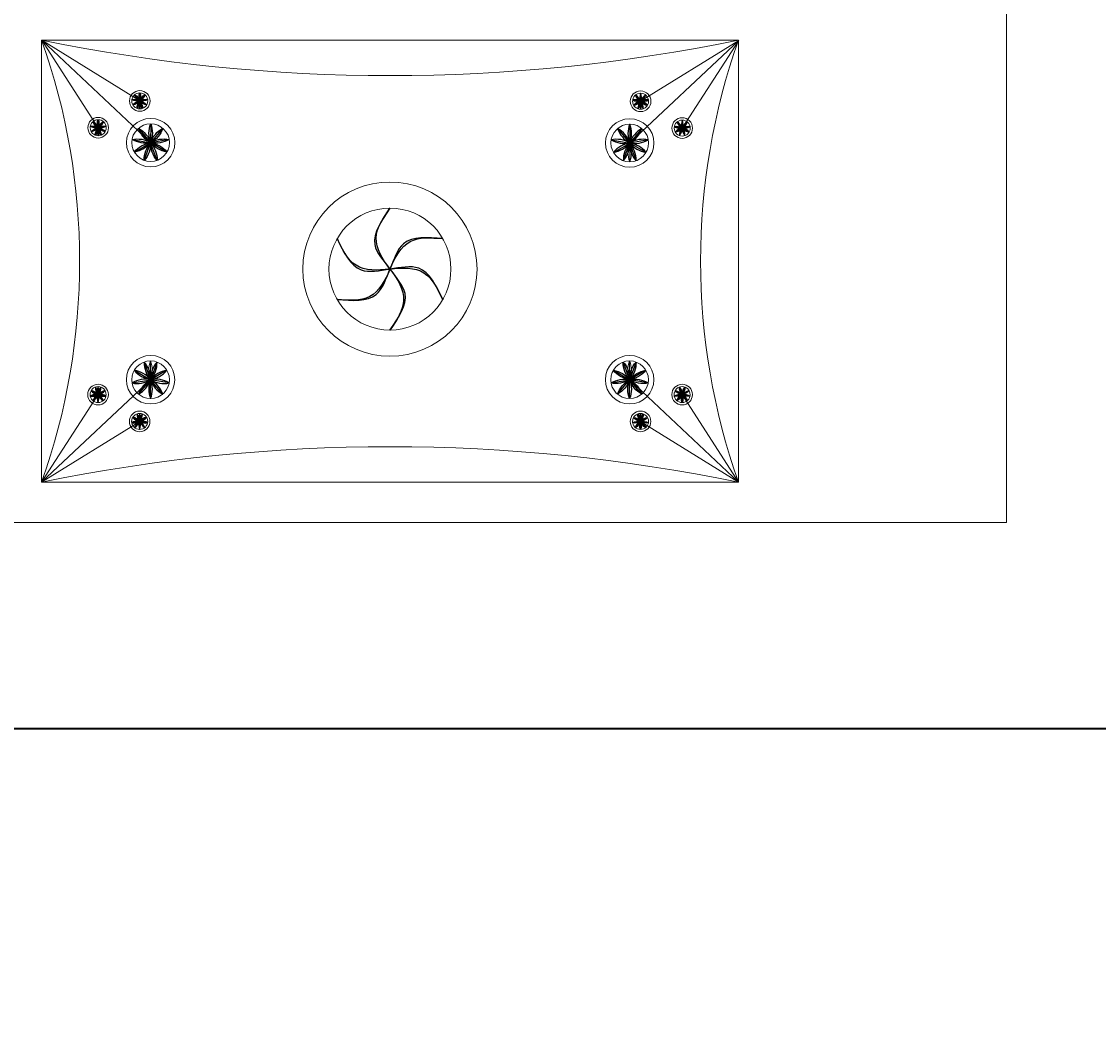
# Model space of a CAD drawing. Units: inches. Extents: x -46 to 1145, y -527 to 760.
# Tile 28 of 57: x 79 to 111, y 222 to 252. Entities that reach past the tile are written whole.
import ezdxf

# ---------------------------------------------------------------- set-up
doc = ezdxf.new("R2010")
doc.units = ezdxf.units.IN
doc.header["$MEASUREMENT"] = 0
for name, color, linetype, lineweight in [('A-ANNO-DIMS', 2, 'Continuous', 18), ('A-FURN', 2, 'Continuous', 13), ('WALLS', 4, 'Continuous', 40)]:
    doc.layers.add(name, color=color, linetype=linetype, lineweight=lineweight)
doc.layers.add('FURNTIURE', color=2, linetype='Continuous')
doc.layers.add('LT', color=9, linetype='Continuous')
doc.styles.get("Standard").update_dxf_attribs({"font": 'arial.ttf'})
doc.dimstyles.get("Standard").update_dxf_attribs({"dimtxt": 0.18, "dimasz": 0.18, "dimexe": 0.18, "dimexo": 0.0625, "dimgap": 0.09, "dimtad": 0, "dimtih": 1, "dimtoh": 1, "dimdec": 0, "dimzin": 0, "dimdsep": 46, "dimlunit": 3, "dimtxsty": 'Standard', "dimcen": 0.09, "dimadec": 0, "dimazin": 0, "dimtfac": 1, "dimtdec": 0, "dimtofl": 0, "dimtmove": 0, "dimatfit": 3, "dimfxl": 1, "dimtolj": 1, "dimtzin": 0, "dimarcsym": 0})

# ---------------------------------------------------------------- blocks, each defined once
blk = doc.blocks.new('*U34')
at = {"layer": 'LT'}
blk.add_line((0, 0.281), (0, -0.281), dxfattribs=at)
for centre, start, end in [((0.734, 0), 159.0676, 200.9324), ((-0.734, 0), 339.0676, 20.9324)]:
    blk.add_arc(centre, 0.786, start, end, dxfattribs=at)
blk = doc.blocks.new('*U35')
at = {"layer": 'LT', "transparency": 16777216}
for p, rotation in [((609.756, 443.96), 40.00000000000002), ((610.117, 443.96), 320), ((609.659, 443.794), 80.00000000000001), ((610.213, 443.794), 280), ((609.693, 443.605), 120), ((609.84, 443.481), 160), ((610.032, 443.481), 200), ((610.179, 443.605), 240)]:
    blk.add_blockref('*U34', p, dxfattribs=dict(at, rotation=rotation))
blk.add_blockref('*U34', (609.936, 444.026), dxfattribs=at)
blk = doc.blocks.new('*U36')
at = {"layer": 'LT'}
blk.add_line((0, 0.12), (0, -0.12), dxfattribs=at)
for centre, start, end in [((0.313, 0), 159.0676, 200.9324), ((-0.313, 0), 339.0676, 20.9324)]:
    blk.add_arc(centre, 0.335, start, end, dxfattribs=at)
blk = doc.blocks.new('*U37')
at = {"layer": 'LT', "transparency": 16777216}
for p, rotation in [((259.536, 188.967), 40), ((259.69, 188.967), 320), ((259.495, 188.896), 80.00000000000001), ((259.509, 188.816), 120), ((259.572, 188.763), 160), ((259.654, 188.763), 200), ((259.716, 188.816), 240), ((259.731, 188.896), 280)]:
    blk.add_blockref('*U36', p, dxfattribs=dict(at, rotation=rotation))
blk.add_blockref('*U36', (259.613, 188.995), dxfattribs=at)
blk = doc.blocks.new('*U38')
at = {"layer": 'LT'}
blk.add_line((0, 0.12), (0, -0.12), dxfattribs=at)
for centre, start, end in [((0.313, 0), 159.0676, 200.9324), ((-0.313, 0), 339.0676, 20.9324)]:
    blk.add_arc(centre, 0.335, start, end, dxfattribs=at)
blk = doc.blocks.new('*U39')
at = {"layer": 'LT', "transparency": 16777216}
for p, rotation in [((259.536, 188.967), 40), ((259.69, 188.967), 320), ((259.495, 188.896), 80.00000000000001), ((259.509, 188.816), 120), ((259.572, 188.763), 160), ((259.654, 188.763), 200), ((259.716, 188.816), 240), ((259.731, 188.896), 280)]:
    blk.add_blockref('*U38', p, dxfattribs=dict(at, rotation=rotation))
blk.add_blockref('*U38', (259.613, 188.995), dxfattribs=at)
blk = doc.blocks.new('*U40')
at = {"layer": 'LT'}
blk.add_line((0, 0.281), (0, -0.281), dxfattribs=at)
for centre, start, end in [((0.734, 0), 159.0676, 200.9324), ((-0.734, 0), 339.0676, 20.9324)]:
    blk.add_arc(centre, 0.786, start, end, dxfattribs=at)
blk = doc.blocks.new('*U41')
at = {"layer": 'LT', "transparency": 16777216}
for p, rotation in [((609.756, 443.96), 40.00000000000002), ((610.117, 443.96), 320), ((609.659, 443.794), 80.00000000000001), ((610.213, 443.794), 280), ((609.693, 443.605), 120), ((609.84, 443.481), 160), ((610.032, 443.481), 200), ((610.179, 443.605), 240)]:
    blk.add_blockref('*U40', p, dxfattribs=dict(at, rotation=rotation))
blk.add_blockref('*U40', (609.936, 444.026), dxfattribs=at)
blk = doc.blocks.new('*U42')
at = {"layer": 'LT'}
blk.add_line((0, 0.12), (0, -0.12), dxfattribs=at)
for centre, start, end in [((0.313, 0), 159.0676, 200.9324), ((-0.313, 0), 339.0676, 20.9324)]:
    blk.add_arc(centre, 0.335, start, end, dxfattribs=at)
blk = doc.blocks.new('*U43')
at = {"layer": 'LT', "transparency": 16777216}
for p, rotation in [((259.536, 188.967), 40), ((259.69, 188.967), 320), ((259.495, 188.896), 80.00000000000001), ((259.509, 188.816), 120), ((259.572, 188.763), 160), ((259.654, 188.763), 200), ((259.716, 188.816), 240), ((259.731, 188.896), 280)]:
    blk.add_blockref('*U42', p, dxfattribs=dict(at, rotation=rotation))
blk.add_blockref('*U42', (259.613, 188.995), dxfattribs=at)
blk = doc.blocks.new('*U44')
at = {"layer": 'LT'}
blk.add_line((0, 0.12), (0, -0.12), dxfattribs=at)
for centre, start, end in [((0.313, 0), 159.0676, 200.9324), ((-0.313, 0), 339.0676, 20.9324)]:
    blk.add_arc(centre, 0.335, start, end, dxfattribs=at)
blk = doc.blocks.new('*U45')
at = {"layer": 'LT', "transparency": 16777216}
for p, rotation in [((259.536, 188.967), 40), ((259.69, 188.967), 320), ((259.495, 188.896), 80.00000000000001), ((259.509, 188.816), 120), ((259.572, 188.763), 160), ((259.654, 188.763), 200), ((259.716, 188.816), 240), ((259.731, 188.896), 280)]:
    blk.add_blockref('*U44', p, dxfattribs=dict(at, rotation=rotation))
blk.add_blockref('*U44', (259.613, 188.995), dxfattribs=at)
blk = doc.blocks.new('*U72')
at = {"layer": 'LT'}
blk.add_line((0, 0.281), (0, -0.281), dxfattribs=at)
for centre, start, end in [((0.734, 0), 159.0676, 200.9324), ((-0.734, 0), 339.0676, 20.9324)]:
    blk.add_arc(centre, 0.786, start, end, dxfattribs=at)
blk = doc.blocks.new('*U73')
at = {"layer": 'LT', "transparency": 16777216}
for p, rotation in [((609.756, 443.96), 40.00000000000002), ((610.117, 443.96), 320), ((609.659, 443.794), 80.00000000000001), ((610.213, 443.794), 280), ((609.693, 443.605), 120), ((609.84, 443.481), 160), ((610.032, 443.481), 200), ((610.179, 443.605), 240)]:
    blk.add_blockref('*U72', p, dxfattribs=dict(at, rotation=rotation))
blk.add_blockref('*U72', (609.936, 444.026), dxfattribs=at)
blk = doc.blocks.new('*U74')
at = {"layer": 'LT'}
blk.add_line((0, 0.12), (0, -0.12), dxfattribs=at)
for centre, start, end in [((0.313, 0), 159.0676, 200.9324), ((-0.313, 0), 339.0676, 20.9324)]:
    blk.add_arc(centre, 0.335, start, end, dxfattribs=at)
blk = doc.blocks.new('*U75')
at = {"layer": 'LT', "transparency": 16777216}
for p, rotation in [((259.536, 188.967), 40), ((259.69, 188.967), 320), ((259.495, 188.896), 80.00000000000001), ((259.509, 188.816), 120), ((259.572, 188.763), 160), ((259.654, 188.763), 200), ((259.716, 188.816), 240), ((259.731, 188.896), 280)]:
    blk.add_blockref('*U74', p, dxfattribs=dict(at, rotation=rotation))
blk.add_blockref('*U74', (259.613, 188.995), dxfattribs=at)
blk = doc.blocks.new('*U76')
at = {"layer": 'LT'}
blk.add_line((0, 0.12), (0, -0.12), dxfattribs=at)
for centre, start, end in [((0.313, 0), 159.0676, 200.9324), ((-0.313, 0), 339.0676, 20.9324)]:
    blk.add_arc(centre, 0.335, start, end, dxfattribs=at)
blk = doc.blocks.new('*U77')
at = {"layer": 'LT', "transparency": 16777216}
for p, rotation in [((259.536, 188.967), 40), ((259.69, 188.967), 320), ((259.495, 188.896), 80.00000000000001), ((259.509, 188.816), 120), ((259.572, 188.763), 160), ((259.654, 188.763), 200), ((259.716, 188.816), 240), ((259.731, 188.896), 280)]:
    blk.add_blockref('*U76', p, dxfattribs=dict(at, rotation=rotation))
blk.add_blockref('*U76', (259.613, 188.995), dxfattribs=at)
blk = doc.blocks.new('*U78')
at = {"layer": 'LT'}
blk.add_line((0, 0.281), (0, -0.281), dxfattribs=at)
for centre, start, end in [((0.734, 0), 159.0676, 200.9324), ((-0.734, 0), 339.0676, 20.9324)]:
    blk.add_arc(centre, 0.786, start, end, dxfattribs=at)
blk = doc.blocks.new('*U79')
at = {"layer": 'LT', "transparency": 16777216}
for p, rotation in [((609.756, 443.96), 40.00000000000002), ((610.117, 443.96), 320), ((609.659, 443.794), 80.00000000000001), ((610.213, 443.794), 280), ((609.693, 443.605), 120), ((609.84, 443.481), 160), ((610.032, 443.481), 200), ((610.179, 443.605), 240)]:
    blk.add_blockref('*U78', p, dxfattribs=dict(at, rotation=rotation))
blk.add_blockref('*U78', (609.936, 444.026), dxfattribs=at)
blk = doc.blocks.new('*U80')
at = {"layer": 'LT'}
blk.add_line((0, 0.12), (0, -0.12), dxfattribs=at)
for centre, start, end in [((0.313, 0), 159.0676, 200.9324), ((-0.313, 0), 339.0676, 20.9324)]:
    blk.add_arc(centre, 0.335, start, end, dxfattribs=at)
blk = doc.blocks.new('*U81')
at = {"layer": 'LT', "transparency": 16777216}
for p, rotation in [((259.536, 188.967), 40), ((259.69, 188.967), 320), ((259.495, 188.896), 80.00000000000001), ((259.509, 188.816), 120), ((259.572, 188.763), 160), ((259.654, 188.763), 200), ((259.716, 188.816), 240), ((259.731, 188.896), 280)]:
    blk.add_blockref('*U80', p, dxfattribs=dict(at, rotation=rotation))
blk.add_blockref('*U80', (259.613, 188.995), dxfattribs=at)
blk = doc.blocks.new('*U82')
at = {"layer": 'LT'}
blk.add_line((0, 0.12), (0, -0.12), dxfattribs=at)
for centre, start, end in [((0.313, 0), 159.0676, 200.9324), ((-0.313, 0), 339.0676, 20.9324)]:
    blk.add_arc(centre, 0.335, start, end, dxfattribs=at)
blk = doc.blocks.new('*U83')
at = {"layer": 'LT', "transparency": 16777216}
for p, rotation in [((259.536, 188.967), 40), ((259.69, 188.967), 320), ((259.495, 188.896), 80.00000000000001), ((259.509, 188.816), 120), ((259.572, 188.763), 160), ((259.654, 188.763), 200), ((259.716, 188.816), 240), ((259.731, 188.896), 280)]:
    blk.add_blockref('*U82', p, dxfattribs=dict(at, rotation=rotation))
blk.add_blockref('*U82', (259.613, 188.995), dxfattribs=at)
blk = doc.blocks.new('*U32')
at = {"layer": 'FURNTIURE'}
blk.add_open_spline([(0.039, 1.82), (-0.218, 1.447), (-0.661, 0.801), (0.102, -0.025), (0.645, -0.928), (0.238, -1.527), (0.039, -1.82)], degree=3, knots=[0, 0, 0, 0, 1.177175, 2.037162, 3.056205, 4.032246, 4.032246, 4.032246, 4.032246], dxfattribs=at)
blk = doc.blocks.new('*U33')
at = {"layer": 'FURNTIURE', "transparency": 16777216}
blk.add_blockref('*U32', (904.302, 663.383), dxfattribs=at)
for p, rotation in [((904.379, 663.383), 180), ((904.321, 663.416), 300), ((904.36, 663.416), 239.9999999999999), ((904.321, 663.349), 59.99999999999999), ((904.36, 663.349), 119.9999999999999)]:
    blk.add_blockref('*U32', p, dxfattribs=dict(at, rotation=rotation))
blk = doc.blocks.new('BED-QUEEN-FURNISHED')
for p, q in [((0, 0), (0, 80)), ((0, 80), (60, 80)), ((8, 78.8), (28.8, 78.8)), ((8, 65.6), (8, 78.8)), ((8, 78.8), (11.385, 75.613)), ((8, 78.8), (9.684, 76.184)), ((8, 78.8), (10.926, 76.984)), ((28.8, 78.8), (25.415, 75.613)), ((28.8, 78.8), (25.874, 76.984)), ((28.8, 78.8), (27.115, 76.184)), ((28.8, 78.8), (28.8, 65.6)), ((10.926, 76.984), (10.926, 76.745)), ((25.874, 76.984), (25.874, 76.745)), ((27.115, 76.184), (27.115, 75.945)), ((11.251, 75.739), (11.251, 75.177)), ((25.548, 75.739), (25.548, 75.177)), ((11.249, 68.673), (11.249, 69.235)), ((7.995, 65.614), (11.382, 68.799)), ((28.795, 65.6), (25.412, 68.789)), ((7.995, 65.614), (9.682, 68.228)), ((27.112, 68.216), (27.113, 68.456)), ((28.795, 65.6), (27.112, 68.216)), ((10.923, 67.428), (10.923, 67.667)), ((25.87, 67.418), (25.87, 67.657)), ((7.995, 65.614), (10.923, 67.428)), ((28.795, 65.6), (25.87, 67.418)), ((8, 65.6), (28.8, 65.6))]:
    blk.add_line(p, q)
for centre, radius in [((10.926, 76.984), 0.308), ((10.926, 76.984), 0.239), ((25.874, 76.984), 0.308), ((25.874, 76.984), 0.239), ((9.684, 76.184), 0.308), ((9.684, 76.184), 0.239), ((11.251, 75.739), 0.723), ((11.251, 75.739), 0.562), ((25.548, 75.739), 0.723), ((25.548, 75.739), 0.562), ((27.115, 76.184), 0.308), ((27.115, 76.184), 0.239), ((18.404, 72.437), 2.599), ((18.404, 72.437), 1.82), ((11.249, 68.673), 0.723), ((11.249, 68.673), 0.562), ((25.546, 68.663), 0.723), ((25.546, 68.663), 0.562), ((9.682, 68.228), 0.308), ((9.682, 68.228), 0.239), ((27.112, 68.216), 0.308), ((27.112, 68.216), 0.239), ((10.923, 67.428), 0.308), ((10.923, 67.428), 0.239), ((25.87, 67.418), 0.308), ((25.87, 67.418), 0.239)]:
    blk.add_circle(centre, radius)
for centre, radius, start, end in [((18.4, 129.177), 51.439, 258.3356, 281.6644), ((-10.654, 72.2), 19.787, 340.5151, 19.4849), ((47.453, 72.2), 19.787, 160.5151, 199.4849), ((11.239, 76.865), 0.335, 159.0676, 200.9324), ((10.614, 76.865), 0.335, 339.0676, 20.9324), ((26.186, 76.865), 0.335, 159.0676, 200.9324), ((25.561, 76.865), 0.335, 339.0676, 20.9324), ((27.428, 76.065), 0.335, 159.0676, 200.9324), ((26.803, 76.065), 0.335, 339.0676, 20.9324), ((11.985, 75.458), 0.786, 159.0676, 200.9324), ((10.517, 75.458), 0.786, 339.0676, 20.9324), ((26.283, 75.458), 0.786, 159.0676, 200.9324), ((24.814, 75.458), 0.786, 339.0676, 20.9324), ((11.983, 68.953), 0.786, 159.028, 200.8928), ((10.515, 68.954), 0.786, 339.028, 20.8928), ((27.425, 68.336), 0.335, 159.028, 200.8928), ((26.8, 68.336), 0.335, 339.028, 20.8928), ((11.235, 67.547), 0.335, 159.028, 200.8928), ((10.61, 67.548), 0.335, 339.028, 20.8928), ((26.183, 67.537), 0.335, 159.028, 200.8928), ((25.558, 67.537), 0.335, 339.028, 20.8928), ((18.4, 15.223), 51.439, 78.3356, 101.6644)]:
    blk.add_arc(centre, radius, start, end)
at = {"xscale": -1}
for name, p in [('*U45', (270.539, -111.891)), ('*U43', (269.297, -112.691)), ('*U41', (621.187, -368.006))]:
    blk.add_blockref(name, p, dxfattribs=at)
for name, p in [('*U39', (-233.739, -111.891)), ('*U35', (-584.388, -368.006)), ('*U37', (-232.498, -112.691)), ('*U33', (-885.936, -590.946))]:
    blk.add_blockref(name, p)
at = {"rotation": 179.9603994254766}
for name, p in [('*U79', (621.491, 511.997)), ('*U81', (269.425, 256.925)), ('*U83', (270.666, 256.124))]:
    blk.add_blockref(name, p, dxfattribs=at)
at = {"xscale": -1, "rotation": 179.9603994254766}
for name, p in [('*U73', (-584.083, 512.83)), ('*U75', (-232.37, 257.271)), ('*U77', (-233.612, 256.472))]:
    blk.add_blockref(name, p, dxfattribs=at)
blk = doc.blocks.new('*D685')
at = {"layer": 'A-ANNO-DIMS', "color": 0, "lineweight": -2, "transparency": 16777216}
for p, q in [((183.501, 700.889), (-46.216, 700.889)), ((-46.036, 700.709), (-46.036, 116.385)), ((-46.036, -468.302), (-46.036, 116.021)), ((12.501, -468.482), (-46.216, -468.482))]:
    blk.add_line(p, q, dxfattribs=at)
at = {"layer": 'A-ANNO-DIMS', "color": 0, "transparency": 16777216}
for points in [[(-46.066, 700.709), (-46.006, 700.709), (-46.036, 700.889)], [(-46.066, -468.302), (-46.006, -468.302), (-46.036, -468.482)]]:
    blk.add_solid(points, dxfattribs=at)
at = {"layer": 'Defpoints', "color": 0, "transparency": 16777216}
for p in [(-46.036, 700.889), (183.564, 700.889), (12.564, -468.482)]:
    blk.add_point(p, dxfattribs=at)
at = {"layer": 'A-ANNO-DIMS', "color": 0, "transparency": 16777216, "insert": (-46.036, 116.203), "char_height": 0.18, "attachment_point": 5}
blk.add_mtext('\\A1;1169.4', dxfattribs=at)

msp = doc.modelspace()

# ---------------------------------------------------------------- linework, layer by layer
at = {"layer": 'WALLS'}
msp.add_line((183.5637, 230.5176), (21.5637, 230.5176), dxfattribs=at)

# ---------------------------------------------------------------- block references
at = {"layer": 'A-FURN', "rotation": 180}
msp.add_blockref('BED-QUEEN-FURNISHED', (108.4877, 316.6818), dxfattribs=at)

# ---------------------------------------------------------------- dimensions: what is measured, and where the dimension line sits
at = {"layer": 'A-ANNO-DIMS'}
dim = msp.add_linear_dim(base=(-46.0363, 700.8886), p1=(12.5637, -468.4824), p2=(183.5637, 700.8886), angle=90, dimstyle='Standard', override={"dimdec": 1, "dimlfac": 1, "dimrnd": 0, "dimzin": 0, "dimdsep": 46, "dimlunit": 2}, dxfattribs=at)
dim.commit()
dim.dimension.update_dxf_attribs({"geometry": '*D685', "text_midpoint": (-46.0363, 116.2031)})

doc.saveas('drawing.dxf')
